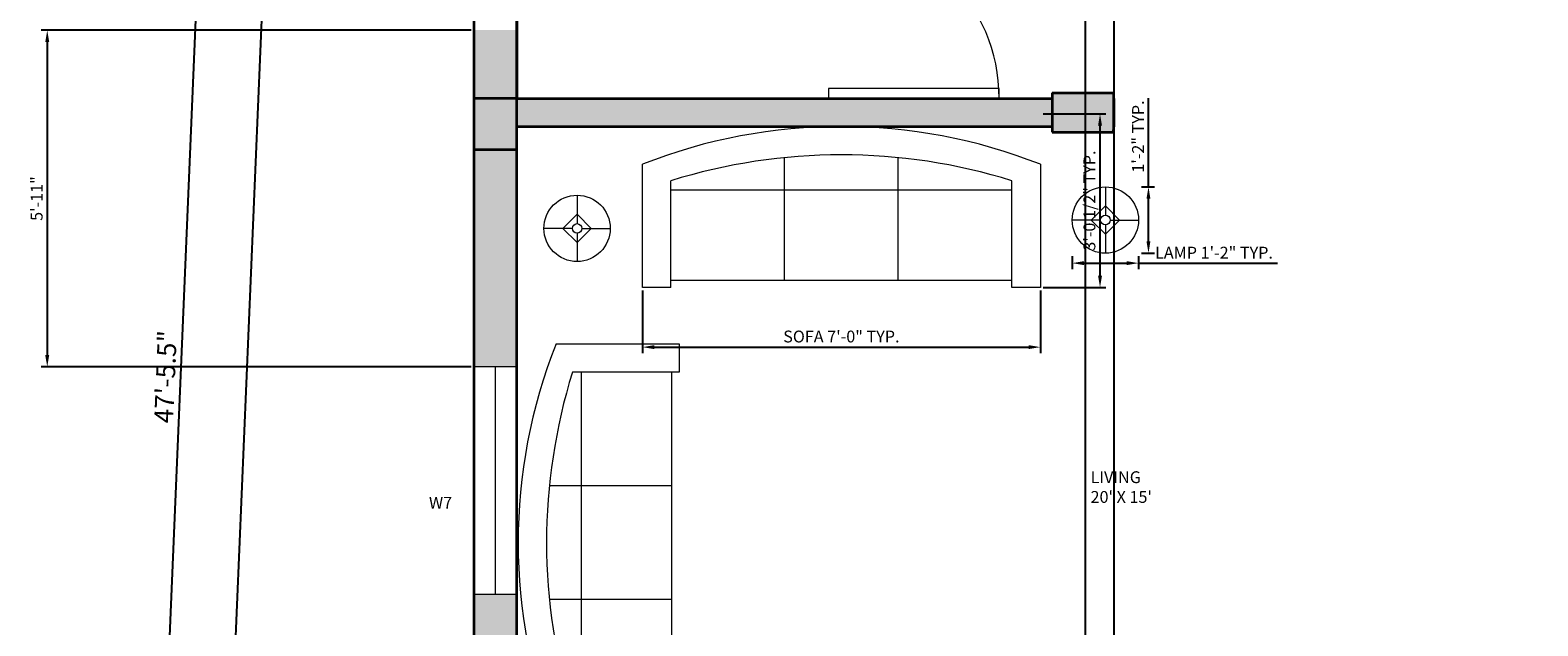
# Model space of a CAD drawing. Units: inches. Extents: x 5395 to 6469, y -203 to 448.
# Tile 2 of 7: x 5397 to 5715, y 78 to 204. Entities that reach past the tile are written whole.
import ezdxf

# ---------------------------------------------------------------- set-up
doc = ezdxf.new("R2010")
doc.units = ezdxf.units.IN
for name, color, linetype, lineweight in [('A-ANNO-DIMS', 2, 'Continuous', 18), ('A-ANNO-TEXT', 6, 'Continuous', 18), ('A-AREA-IDEN', 6, 'Continuous', 18), ('A-COLS', 7, 'Continuous', 35), ('A-COLS-PATT', 2, 'Continuous', 13), ('A-GLAZ', 4, 'Continuous', 18), ('A-WALL', 7, 'Continuous', 35), ('A-WALL-PATT', 11, 'Continuous', 9), ('C-PROP', 7, 'Continuous', 25), ('door', 240, 'Continuous', 18), ('furniture', 70, 'Continuous', 18)]:
    doc.layers.add(name, color=color, linetype=linetype, lineweight=lineweight)
doc.styles.get("Standard").update_dxf_attribs({"font": 'arial.ttf'})
doc.dimstyles.new('ISO-25', dxfattribs={"dimtxt": 2.5, "dimasz": 2.5, "dimexe": 1.25, "dimexo": 0.625, "dimtad": 1, "dimdec": 1, "dimlunit": 3, "dimtxsty": 'Standard', "dimcen": 2.5, "dimadec": 0, "dimazin": 0, "dimtfac": 1, "dimtdec": 1, "dimtmove": 0, "dimatfit": 3, "dimfxl": 1, "dimarcsym": 0})

# ---------------------------------------------------------------- blocks, each defined once
blk = doc.blocks.new('*U4')
for p, q in [((0, 0), (0, 5)), ((30, 0), (30, 5))]:
    blk.add_line(p, q)
blk.add_lwpolyline([(0, 0), (0, -30), (1.75, -30), (1.75, 0)], close=True)
blk.add_arc((0, 0), 30, 270, 0)
blk = doc.blocks.new('Sofa - Roundback 7 ft.')
for p, q in [((-12.00002, -32.4421), (-12.00003, -6.5971)), ((11.99997, -32.4421), (11.99998, -6.5971)), ((-36.000027, -34), (-36.000027, -11.4696)), ((35.99998, -34), (35.99998, -11.4696)), ((-35.999844, -13.3819), (35.9998, -13.3819)), ((-36.000027, -32.4421), (35.99998, -32.4421))]:
    blk.add_line(p, q)
for points in [[(-36.000027, -34), (-42.000027, -34), (-42.000027, -8)], [(41.99998, -8), (41.99998, -34), (35.99998, -34)]]:
    blk.add_lwpolyline(points)
for centre, radius, start, end in [((0, -114.25), 114.25, 68.43141, 111.5686), ((-0.00001, -127.1968), 121.1968, 72.72033, 107.2797)]:
    blk.add_arc(centre, radius, start, end)
blk = doc.blocks.new('Lamp - Table')
for p, q in [((0, 7), (0, 1)), ((-1, 0), (-7, 0)), ((0, 3), (-3, 0)), ((-3, 0), (0, -3)), ((3, 0), (0, 3)), ((0, -3), (3, 0)), ((1, 0), (7, 0)), ((0, -1), (0, -7))]:
    blk.add_line(p, q)
for radius in [7, 1]:
    blk.add_circle((0, 0), radius)
blk = doc.blocks.new('*D20')
at = {"layer": 'A-ANNO-DIMS', "color": 0, "lineweight": -2, "transparency": 16777216}
for p, q in [((5454.31, 414.33), (5439.73, 414.95)), ((5440.87, 412.4), (5417.08, -151.61)), ((5430.31, -154.67), (5415.73, -154.05))]:
    blk.add_line(p, q, dxfattribs=at)
at = {"layer": 'A-ANNO-DIMS', "color": 0, "transparency": 16777216}
for points in [[(5440.46, 412.41), (5441.29, 412.38), (5440.98, 414.89)], [(5416.67, -151.59), (5417.5, -151.63), (5416.98, -154.11)]]:
    blk.add_solid(points, dxfattribs=at)
at = {"layer": 'Defpoints', "color": 0, "transparency": 16777216}
for p in [(5454.94, 414.31), (5416.98, -154.11), (5430.94, -154.69)]:
    blk.add_point(p, dxfattribs=at)
at = {"layer": 'A-ANNO-DIMS', "color": 0, "transparency": 16777216, "insert": (5426.32, 130.51), "char_height": 4, "attachment_point": 5, "rotation": 87.5847}
blk.add_mtext('47\'-5.5"', dxfattribs=at)
blk = doc.blocks.new('WINDOW-48IN')
for p, q in [((0, 0), (0, 9)), ((48, 0), (48, 9)), ((0, 4.5), (48, 4.5))]:
    blk.add_line(p, q)
blk = doc.blocks.new('*D41')
at = {"layer": 'A-ANNO-DIMS', "color": 0, "lineweight": -2, "transparency": 16777216}
for p, q in [((5526.46, 148.76), (5526.46, 135.53)), ((5610.46, 148.76), (5610.46, 135.53)), ((5528.96, 136.78), (5607.96, 136.78))]:
    blk.add_line(p, q, dxfattribs=at)
at = {"layer": 'A-ANNO-DIMS', "color": 0, "transparency": 16777216}
for points in [[(5528.96, 137.2), (5528.96, 136.37), (5526.46, 136.78)], [(5607.96, 137.2), (5607.96, 136.37), (5610.46, 136.78)]]:
    blk.add_solid(points, dxfattribs=at)
at = {"layer": 'Defpoints', "color": 0, "transparency": 16777216}
for p in [(5526.46, 149.38), (5610.46, 149.38), (5610.46, 136.78)]:
    blk.add_point(p, dxfattribs=at)
at = {"layer": 'A-ANNO-DIMS', "color": 0, "transparency": 16777216, "insert": (5568.46, 138.7), "char_height": 2.5, "attachment_point": 5}
blk.add_mtext('SOFA 7\'-0" TYP.', dxfattribs=at)
blk = doc.blocks.new('*D42')
at = {"layer": 'A-ANNO-DIMS', "color": 0, "lineweight": -2, "transparency": 16777216}
for p, q in [((5611.08, 186.05), (5624.31, 186.05)), ((5623.06, 151.88), (5623.06, 183.55)), ((5611.08, 149.38), (5624.31, 149.38))]:
    blk.add_line(p, q, dxfattribs=at)
at = {"layer": 'A-ANNO-DIMS', "color": 0, "transparency": 16777216}
for points in [[(5622.64, 183.55), (5623.47, 183.55), (5623.06, 186.05)], [(5622.64, 151.88), (5623.47, 151.88), (5623.06, 149.38)]]:
    blk.add_solid(points, dxfattribs=at)
at = {"layer": 'Defpoints', "color": 0, "transparency": 16777216}
for p in [(5610.46, 186.05), (5623.06, 186.05), (5610.46, 149.38)]:
    blk.add_point(p, dxfattribs=at)
at = {"layer": 'A-ANNO-DIMS', "color": 0, "transparency": 16777216, "insert": (5621.14, 167.72), "char_height": 2.5, "attachment_point": 5, "rotation": 90}
blk.add_mtext('3\'-0 1/2" TYP.', dxfattribs=at)
blk = doc.blocks.new('*D47')
at = {"layer": 'A-ANNO-DIMS', "color": 0, "lineweight": -2, "transparency": 16777216}
for p, q in [((5617.18, 155.99), (5617.18, 153.27)), ((5631.18, 155.99), (5631.18, 153.27)), ((5619.68, 154.52), (5628.68, 154.52)), ((5631.18, 154.52), (5660.54, 154.52))]:
    blk.add_line(p, q, dxfattribs=at)
at = {"layer": 'A-ANNO-DIMS', "color": 0, "transparency": 16777216}
for points in [[(5619.68, 154.93), (5619.68, 154.1), (5617.18, 154.52)], [(5628.68, 154.93), (5628.68, 154.1), (5631.18, 154.52)]]:
    blk.add_solid(points, dxfattribs=at)
at = {"layer": 'Defpoints', "color": 0, "transparency": 16777216}
for p in [(5617.18, 156.62), (5631.18, 156.62), (5631.18, 154.52)]:
    blk.add_point(p, dxfattribs=at)
at = {"layer": 'A-ANNO-DIMS', "color": 0, "transparency": 16777216, "insert": (5647.11, 156.4), "char_height": 2.5, "attachment_point": 5}
blk.add_mtext('LAMP 1\'-2" TYP.', dxfattribs=at)
blk = doc.blocks.new('*D48')
at = {"layer": 'A-ANNO-DIMS', "color": 0, "lineweight": -2, "transparency": 16777216}
for p, q in [((5633.28, 170.62), (5633.28, 189.37)), ((5631.8, 170.62), (5634.53, 170.62)), ((5633.28, 159.12), (5633.28, 168.12)), ((5631.8, 156.62), (5634.53, 156.62))]:
    blk.add_line(p, q, dxfattribs=at)
at = {"layer": 'A-ANNO-DIMS', "color": 0, "transparency": 16777216}
for points in [[(5632.86, 168.12), (5633.69, 168.12), (5633.28, 170.62)], [(5632.86, 159.12), (5633.69, 159.12), (5633.28, 156.62)]]:
    blk.add_solid(points, dxfattribs=at)
at = {"layer": 'Defpoints', "color": 0, "transparency": 16777216}
for p in [(5631.18, 170.62), (5633.28, 170.62), (5631.18, 156.62)]:
    blk.add_point(p, dxfattribs=at)
at = {"layer": 'A-ANNO-DIMS', "color": 0, "transparency": 16777216, "insert": (5631.4, 181.24), "char_height": 2.5, "attachment_point": 5, "rotation": 90}
blk.add_mtext('1\'-2" TYP.', dxfattribs=at)
blk = doc.blocks.new('*D66')
at = {"layer": 'A-ANNO-DIMS', "color": 0, "lineweight": -2, "transparency": 16777216}
for p, q in [((5490.31, 203.71), (5399.59, 203.71)), ((5400.84, 201.21), (5400.84, 135.09)), ((5490.31, 132.59), (5399.59, 132.59))]:
    blk.add_line(p, q, dxfattribs=at)
at = {"layer": 'A-ANNO-DIMS', "color": 0, "transparency": 16777216}
for points in [[(5400.42, 201.21), (5401.25, 201.21), (5400.84, 203.71)], [(5400.42, 135.09), (5401.25, 135.09), (5400.84, 132.59)]]:
    blk.add_solid(points, dxfattribs=at)
at = {"layer": 'Defpoints', "color": 0, "transparency": 16777216}
for p in [(5490.94, 203.71), (5400.84, 132.59), (5490.94, 132.59)]:
    blk.add_point(p, dxfattribs=at)
at = {"layer": 'A-ANNO-DIMS', "color": 0, "transparency": 16777216, "insert": (5398.93, 168.15), "char_height": 2.5, "attachment_point": 5, "rotation": 90}
blk.add_mtext('5\'-11"', dxfattribs=at)
blk = doc.blocks.new('*D72')
at = {"layer": 'A-ANNO-DIMS', "color": 0, "lineweight": -2, "transparency": 16777216}
for p, q in [((5619.94, 236.68), (5619.94, -186.04)), ((5625.94, 236.68), (5625.94, -186.04)), ((5617.44, -184.79), (5614.94, -184.79)), ((5619.94, -184.79), (5625.94, -184.79)), ((5628.44, -184.79), (5638.83, -184.79))]:
    blk.add_line(p, q, dxfattribs=at)
at = {"layer": 'A-ANNO-DIMS', "color": 0, "transparency": 16777216}
for points in [[(5617.44, -184.38), (5617.44, -185.21), (5619.94, -184.79)], [(5628.44, -184.38), (5628.44, -185.21), (5625.94, -184.79)]]:
    blk.add_solid(points, dxfattribs=at)
at = {"layer": 'Defpoints', "color": 0, "transparency": 16777216}
for p in [(5619.94, 237.31), (5625.94, 237.31), (5625.94, -184.79)]:
    blk.add_point(p, dxfattribs=at)
at = {"layer": 'A-ANNO-DIMS', "color": 0, "transparency": 16777216, "insert": (5634.88, -182.89), "char_height": 2.5, "attachment_point": 5}
blk.add_mtext('0\'-6"', dxfattribs=at)

msp = doc.modelspace()

# ---------------------------------------------------------------- hatches: boundary and pattern name
at = {"layer": 'A-COLS-PATT'}
h = msp.add_hatch(color=256, dxfattribs=at)
h.dxf.hatch_style = 1
h.paths.add_polyline_path([(5499.94, 189.31), (5490.94, 189.31), (5490.94, 178.42), (5499.94, 178.42)])
h = msp.add_hatch(color=256, dxfattribs=at)
h.dxf.hatch_style = 1
h.paths.add_polyline_path([(5625.94, 190.46), (5612.93, 190.46), (5612.93, 182.2), (5625.93, 182.2), (5625.94, 183.31)])
at = {"layer": 'A-WALL-PATT'}
h = msp.add_hatch(color=256, dxfattribs=at)
h.dxf.hatch_style = 1
h.paths.add_polyline_path([(5538.88, 378.31), (5499.94, 378.31), (5499.94, 369.31), (5538.88, 369.31)])
h.paths.add_polyline_path([(5499.94, 276.14), (5490.94, 276.14), (5490.94, 227.71), (5499.94, 227.71), (5499.94, 237.31)])
h.paths.add_polyline_path([(5565.94, 243.31), (5499.94, 243.31), (5499.94, 237.31), (5559.94, 237.31), (5559.94, 225.31), (5565.94, 225.31)])
h.paths.add_polyline_path([(5625.94, 367.55), (5619.94, 367.55), (5619.94, 237.31), (5625.94, 237.31)])
h.paths.add_polyline_path([(5745.94, 369.31), (5739.94, 369.31), (5739.94, 237.31), (5745.94, 237.31)])
h.paths.add_polyline_path([(5745.94, 192.25), (5739.94, 192.25), (5739.94, 190.23), (5745.94, 190.23)])
h.paths.add_polyline_path([(5745.94, 180.33), (5739.94, 180.33), (5739.94, 47.04), (5745.94, 47.04)])
h.paths.add_polyline_path([(5877.94, 183.31), (5884.03, 183.31), (5884.03, 189.31), (5747.34, 189.31), (5747.34, 183.31), (5871.94, 183.31), (5871.94, 82.27), (5877.94, 82.27), (5877.94, 90.31), (5925.94, 90.31), (5925.94, 96.31), (5877.94, 96.31)])
h.paths.add_polyline_path([(5934.94, 128.85), (5925.94, 128.85), (5925.94, 55.61), (5934.94, 55.61)])
h.paths.add_polyline_path([(5934.94, 181.4), (5925.94, 181.4), (5925.94, 152.85), (5934.94, 152.85)])
h.paths.add_polyline_path([(5925.94, 189.31), (5914.03, 189.31), (5914.03, 183.31), (5925.94, 183.31)], flags=17)
h.paths.add_polyline_path([(5934.94, 369.31), (5925.94, 369.31), (5925.94, 237.31), (5934.94, 237.31)])
h.paths.add_polyline_path([(5657.93, 378.31), (5627.19, 378.31), (5627.19, 369.31), (5657.93, 369.31)])
h.paths.add_polyline_path([(5619.94, 378.31), (5586.88, 378.31), (5586.88, 369.31), (5619.94, 369.31)])
h.paths.add_polyline_path([(5739.94, 378.31), (5705.93, 378.31), (5705.93, 369.31), (5739.94, 369.31)])
h.paths.add_polyline_path([(5812.1, 378.31), (5753.55, 378.31), (5753.55, 369.31), (5812.1, 369.31)])
h.paths.add_polyline_path([(5923.7, 378.31), (5860.1, 378.31), (5860.1, 369.31), (5923.7, 369.31)])
h.paths.add_polyline_path([(5499.94, 203.71), (5490.94, 203.71), (5490.94, 189.31), (5499.94, 189.31)])
h.paths.add_polyline_path([(5612.93, 189.31), (5499.94, 189.31), (5499.94, 183.31), (5612.93, 183.31)])
h.paths.add_polyline_path([(5499.94, 178.42), (5490.94, 178.42), (5490.94, 132.59), (5499.94, 132.59)])
h.paths.add_polyline_path([(5499.94, 84.59), (5490.94, 84.59), (5490.94, 47.04), (5499.94, 47.04)])
h.paths.add_polyline_path([(5499.94, 11.04), (5490.94, 11.04), (5490.94, 3.31), (5499.94, 3.31)])
h.paths.add_polyline_path([(5532.25, 3.31), (5502.78, 3.31), (5502.78, -5.69), (5532.25, -5.69)])
h.paths.add_polyline_path([(5601.84, 3.31), (5580.25, 3.31), (5580.25, -5.69), (5601.84, -5.69)])
h.paths.add_polyline_path([(5625.94, 3.31), (5614.13, 3.31), (5614.13, -5.69), (5625.94, -5.69)])
h.paths.add_polyline_path([(5787.9, 3.31), (5748.46, 3.31), (5748.46, -5.69), (5787.9, -5.69)])
h.paths.add_polyline_path([(5737.31, 3.31), (5697.94, 3.31), (5697.94, -5.69), (5737.31, -5.69)])
h.paths.add_polyline_path([(5745.94, 11.04), (5739.94, 11.04), (5739.94, 3.31), (5745.94, 3.31)])
h.paths.add_polyline_path([(5922.21, 3.31), (5877.94, 3.31), (5877.94, 46.27), (5871.94, 46.27), (5871.94, 3.31), (5835.9, 3.31), (5835.9, -5.69), (5922.21, -5.69)])
h.paths.add_polyline_path([(5934.94, 31.61), (5925.94, 31.61), (5925.94, 3.31), (5934.94, 3.31)])

# ---------------------------------------------------------------- linework, layer by layer
at = {"layer": 'A-COLS'}
for p, q in [((5499.94, 189.31), (5490.94, 189.31)), ((5612.93, 190.46), (5612.93, 182.2)), ((5612.93, 190.46), (5625.94, 190.46)), ((5625.94, 183.31), (5625.94, 190.46)), ((5612.93, 182.2), (5625.93, 182.2)), ((5625.93, 182.2), (5625.94, 183.31)), ((5499.94, 178.42), (5490.94, 178.42))]:
    msp.add_line(p, q, dxfattribs=at)
at = {"layer": 'A-WALL'}
for p, q in [((5490.94, 47.04), (5490.94, 378.31)), ((5499.94, 47.04), (5499.94, 369.31)), ((5499.94, 189.31), (5612.93, 189.31)), ((5625.94, 189.31), (5625.94, 183.31)), ((5612.93, 183.31), (5499.94, 183.31))]:
    msp.add_line(p, q, dxfattribs=at)
msp.add_lwpolyline([(5499.94, 237.31), (5499.94, 189.31)], dxfattribs=at)
at = {"layer": 'C-PROP'}
msp.add_line((5430.94, -154.69), (5454.94, 414.31), dxfattribs=at)

# ---------------------------------------------------------------- block references
at = {"layer": 'A-GLAZ', "rotation": 89.99999999999699}
msp.add_blockref('WINDOW-48IN', (5499.94, 84.59), dxfattribs=at)
at = {"layer": 'door', "xscale": 1.200014089153335, "yscale": 1.200014089153335, "zscale": 1.200014089153335, "rotation": 90}
msp.add_blockref('*U4', (5565.76, 189.31), dxfattribs=at)
at = {"layer": 'furniture'}
for name, p in [('Sofa - Roundback 7 ft.', (5568.46, 183.38)), ('Lamp - Table', (5512.68, 161.85)), ('Lamp - Table', (5624.18, 163.62))]:
    msp.add_blockref(name, p, dxfattribs=at)
at = {"layer": 'furniture', "rotation": 90}
msp.add_blockref('Sofa - Roundback 7 ft.', (5500.23, 95.49), dxfattribs=at)

# ---------------------------------------------------------------- texts
at = {"layer": 'A-ANNO-TEXT', "insert": (5481.41, 105.17), "char_height": 2.5, "attachment_point": 1}
msp.add_mtext_dynamic_manual_height_columns('W7', width=62.1492, gutter_width=12.5, heights=[0], dxfattribs=at)
at = {"layer": 'A-AREA-IDEN', "insert": (5621.06, 110.57), "char_height": 2.5, "attachment_point": 1}
msp.add_mtext_dynamic_manual_height_columns("LIVING\\P20' X 15'", width=62.1492, gutter_width=12.5, heights=[0], dxfattribs=at)

# ---------------------------------------------------------------- dimensions: what is measured, and where the dimension line sits
at = {"layer": 'A-ANNO-DIMS'}
dim = msp.add_aligned_dim(p1=(5454.94, 414.31), p2=(5430.94, -154.69), distance=-13.97, dimstyle='ISO-25', override={"dimtxt": 4, "dimclrd": 0, "dimclre": 0, "dimclrt": 0}, dxfattribs=at)
dim.commit()
dim.dimension.update_dxf_attribs({"geometry": '*D20', "text_midpoint": (5426.32, 130.51)})
dim = msp.add_linear_dim(base=(5625.94, -184.79), p1=(5619.94, 237.31), p2=(5625.94, 237.31), dimstyle='ISO-25', override={"dimdec": 1, "dimlfac": 1, "dimrnd": 0, "dimzin": 1, "dimdsep": 46, "dimlunit": 4, "dimfrac": 2}, dxfattribs=at)
dim.commit()
dim.dimension.update_dxf_attribs({"geometry": '*D72', "text_midpoint": (5634.88, -182.89)})
dim = msp.add_linear_dim(base=(5400.84, 132.59), p1=(5490.94, 203.71), p2=(5490.94, 132.59), angle=90, dimstyle='ISO-25', override={"dimdec": 1, "dimlfac": 1, "dimrnd": 0, "dimzin": 1, "dimdsep": 46, "dimlunit": 4, "dimfrac": 2}, dxfattribs=at)
dim.commit()
dim.dimension.update_dxf_attribs({"geometry": '*D66', "text_midpoint": (5398.93, 168.15)})
for base, p1, p2, picture, middle in [((5633.28, 170.62), (5631.18, 156.62), (5631.18, 170.62), '*D48', (5631.4, 181.24)), ((5623.06, 186.05), (5610.46, 149.38), (5610.46, 186.05), '*D42', (5621.14, 167.72))]:
    dim = msp.add_linear_dim(base=base, p1=p1, p2=p2, angle=90, text='<> TYP.', dimstyle='ISO-25', override={"dimdec": 1, "dimlfac": 1, "dimrnd": 0, "dimzin": 1, "dimdsep": 46, "dimlunit": 4, "dimfrac": 2}, dxfattribs=at)
    dim.commit()
    dim.dimension.update_dxf_attribs({"geometry": picture, "text_midpoint": middle})
for base, p1, p2, text, picture, middle in [((5631.18, 154.52), (5617.18, 156.62), (5631.18, 156.62), 'LAMP <> TYP.', '*D47', (5647.11, 156.4)), ((5610.46, 136.78), (5526.46, 149.38), (5610.46, 149.38), 'SOFA <> TYP.', '*D41', (5568.46, 138.7))]:
    dim = msp.add_linear_dim(base=base, p1=p1, p2=p2, text=text, dimstyle='ISO-25', override={"dimdec": 1, "dimlfac": 1, "dimrnd": 0, "dimzin": 1, "dimdsep": 46, "dimlunit": 4, "dimfrac": 2}, dxfattribs=at)
    dim.commit()
    dim.dimension.update_dxf_attribs({"geometry": picture, "text_midpoint": middle})

doc.saveas('drawing.dxf')
